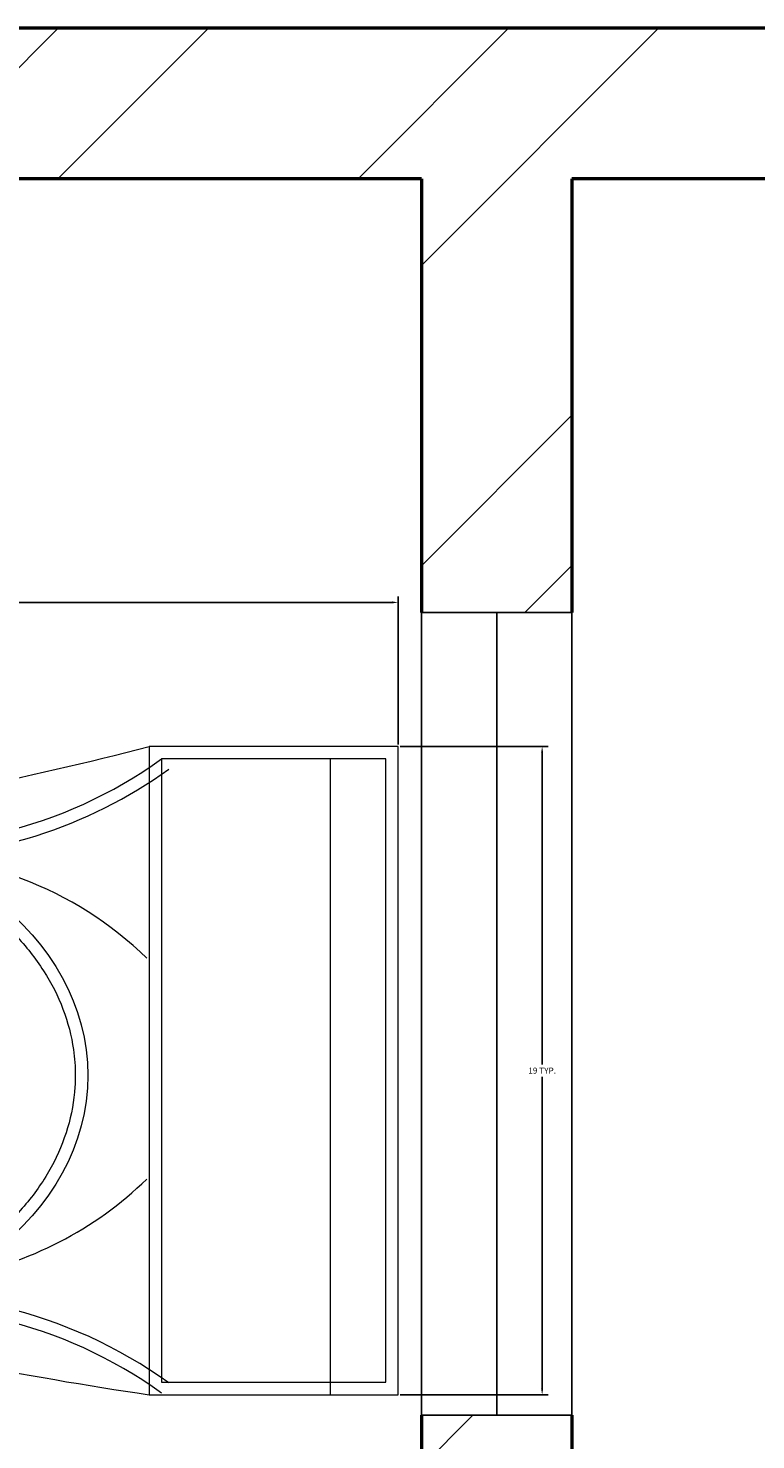
# Model space of a CAD drawing. Units: inches. Extents: x 963 to 2075, y 289 to 2657.
# Tile 35 of 98: x 1668 to 1689, y 1505 to 1547. Entities that reach past the tile are written whole.
import ezdxf

# ---------------------------------------------------------------- set-up
doc = ezdxf.new("R2010")
doc.units = ezdxf.units.IN
for name, color, linetype, lineweight in [('A-ANNO-DIMS', 2, 'Continuous', 18), ('A-FLOR-FIXT', 9, 'Continuous', 18), ('A-GLAZ', 3, 'Continuous', 25), ('A-WALL', 7, 'Continuous', 50), ('A-WALL-PATT', 8, 'Continuous', 13)]:
    doc.layers.add(name, color=color, linetype=linetype, lineweight=lineweight)
doc.styles.get("Standard").update_dxf_attribs({"font": 'arial.ttf'})
doc.dimstyles.get("Standard").update_dxf_attribs({"dimtxt": 0.18, "dimasz": 0.18, "dimexe": 0.18, "dimexo": 0.0625, "dimgap": 0.09, "dimtad": 0, "dimtih": 1, "dimtoh": 1, "dimdec": 4, "dimzin": 0, "dimdsep": 46, "dimtxsty": 'Standard', "dimcen": 0.09, "dimadec": 0, "dimazin": 0, "dimtfac": 1, "dimtdec": 4, "dimtofl": 0, "dimtmove": 0, "dimatfit": 3, "dimfxl": 1, "dimtolj": 1, "dimtzin": 0, "dimarcsym": 0})

# ---------------------------------------------------------------- blocks, each defined once
blk = doc.blocks.new('A$C31115884')
for p, q in [((257.5, 466.4), (257.5, 523.2)), ((283.1, 497.7), (223.4, 497.7)), ((0, 200), (0, 0)), ((520, 200), (0, 200)), ((520, 0), (520, 200)), ((10, 190), (10, 10)), ((510, 190), (10, 190)), ((510, 10), (510, 190)), ((510, 54.5), (0, 54.5)), ((10, 10), (510, 10)), ((0, 0), (520, 0))]:
    blk.add_line(p, q)
blk.add_circle((255.6, 496.4), 23.6)
for centre, radius, start, end in [((2777.7, -204.6), 2807, 165.4549, 171.7133), ((3237, 905), 2807, 188.2867, 194.5451), ((-294.5, 403.3), 364.7, 324.2091, 9.3499), ((-294.5, 403.3), 374.7, 324.2091, 9.3499), ((805.8, 403.3), 364.7, 170.6501, 215.7909), ((139.5, 406.2), 293.5, 315.8436, 2.6563), ((805.8, 403.3), 374.7, 179.2036, 215.7909), ((383.6, 406.2), 293.5, 190.2774, 224.1564)]:
    blk.add_arc(centre, radius, start, end)
blk.add_ellipse((256.2, 509.9), major_axis=(0, -260.7), ratio=0.772727)
blk.add_open_spline([(256.2, 259.2), (263.1, 259.2), (270, 259.7), (287.8, 262.3), (298.7, 265.1), (319.9, 273.1), (330.2, 278.4), (350.1, 291.1), (359.7, 298.7), (377.7, 315.9), (386.2, 325.5), (401.7, 346.6), (408.8, 358.1), (421.3, 382.5), (426.8, 395.5), (435.9, 422.4), (439.5, 436.4), (444.8, 465.1), (446.5, 479.7), (447.9, 509.2), (447.6, 524), (445, 553.3), (442.7, 567.8), (436.3, 596), (432.1, 609.7), (421.9, 636), (416, 648.6), (402.5, 672.1), (395, 683), (378.6, 703), (369.8, 712.1), (351.1, 728), (341.3, 734.8), (320.9, 746.2), (310.4, 750.7), (288.9, 757.3), (278, 759.4), (256, 761), (245, 760.6), (223.1, 757.2), (212.3, 754.3), (191.1, 746.1), (180.8, 740.7), (160.9, 727.8), (151.4, 720.1), (133.5, 702.7), (125.1, 693), (109.6, 671.7), (102.6, 660.2), (90.2, 635.7), (84.9, 622.7), (76, 595.6), (72.4, 581.6), (67.2, 552.9), (65.6, 538.2), (64.4, 508.8), (64.8, 494), (67.5, 464.7), (69.9, 450.2), (76.6, 422), (80.8, 408.3), (91.1, 382.2), (97.2, 369.7), (110.8, 346.3), (118.4, 335.4), (134.8, 315.6), (143.7, 306.7), (162.4, 290.9), (172.3, 284.2), (192.8, 273), (203.3, 268.6), (224.8, 262.2), (235.8, 260.2), (249.9, 259.3), (253, 259.2), (256.2, 259.2)], degree=3, knots=[0, 0, 0, 0, 0.110105, 0.110105, 0.285049, 0.285049, 0.459994, 0.459994, 0.634938, 0.634938, 0.809882, 0.809882, 0.984827, 0.984827, 1.159771, 1.159771, 1.334715, 1.334715, 1.50966, 1.50966, 1.684604, 1.684604, 1.859549, 1.859549, 2.034493, 2.034493, 2.209437, 2.209437, 2.384382, 2.384382, 2.559326, 2.559326, 2.73427, 2.73427, 2.909215, 2.909215, 3.084159, 3.084159, 3.259103, 3.259103, 3.434048, 3.434048, 3.608992, 3.608992, 3.783936, 3.783936, 3.958881, 3.958881, 4.133825, 4.133825, 4.30877, 4.30877, 4.483714, 4.483714, 4.658658, 4.658658, 4.833603, 4.833603, 5.008547, 5.008547, 5.183491, 5.183491, 5.358436, 5.358436, 5.53338, 5.53338, 5.708324, 5.708324, 5.883269, 5.883269, 6.058213, 6.058213, 6.233158, 6.233158, 6.283185, 6.283185, 6.283185, 6.283185])
blk = doc.blocks.new('*D16')
at = {"layer": 'A-ANNO-DIMS', "color": 0, "lineweight": -2, "transparency": 16777216}
for p, q in [((1650.002, 1525.905), (1650.002, 1530.33)), ((1678.722, 1525.905), (1678.722, 1530.33)), ((1650.182, 1530.15), (1663.586, 1530.15)), ((1678.542, 1530.15), (1665.138, 1530.15))]:
    blk.add_line(p, q, dxfattribs=at)
at = {"layer": 'A-ANNO-DIMS', "color": 0, "transparency": 16777216}
for points in [[(1650.182, 1530.18), (1650.182, 1530.12), (1650.002, 1530.15)], [(1678.542, 1530.18), (1678.542, 1530.12), (1678.722, 1530.15)]]:
    blk.add_solid(points, dxfattribs=at)
at = {"layer": 'Defpoints', "color": 0, "transparency": 16777216}
for p in [(1650.002, 1530.15), (1650.002, 1525.842), (1678.722, 1525.842)]:
    blk.add_point(p, dxfattribs=at)
at = {"layer": 'A-ANNO-DIMS', "color": 0, "transparency": 16777216, "insert": (1664.362, 1530.15), "char_height": 0.18, "attachment_point": 5}
blk.add_mtext('\\A1;WC 29 TYP.', dxfattribs=at)
blk = doc.blocks.new('*D17')
at = {"layer": 'A-ANNO-DIMS', "color": 0, "lineweight": -2, "transparency": 16777216}
for p, q in [((1678.785, 1525.842), (1683.21, 1525.842)), ((1683.03, 1525.662), (1683.03, 1516.334)), ((1683.03, 1506.641), (1683.03, 1515.97)), ((1678.785, 1506.461), (1683.21, 1506.461))]:
    blk.add_line(p, q, dxfattribs=at)
at = {"layer": 'A-ANNO-DIMS', "color": 0, "transparency": 16777216}
for points in [[(1683, 1525.662), (1683.06, 1525.662), (1683.03, 1525.842)], [(1683, 1506.641), (1683.06, 1506.641), (1683.03, 1506.461)]]:
    blk.add_solid(points, dxfattribs=at)
at = {"layer": 'Defpoints', "color": 0, "transparency": 16777216}
for p in [(1678.722, 1525.842), (1683.03, 1525.842), (1678.722, 1506.461)]:
    blk.add_point(p, dxfattribs=at)
at = {"layer": 'A-ANNO-DIMS', "color": 0, "transparency": 16777216, "insert": (1683.03, 1516.152), "char_height": 0.18, "attachment_point": 5}
blk.add_mtext('\\A1;19 TYP.', dxfattribs=at)

msp = doc.modelspace()

# ---------------------------------------------------------------- hatches: boundary and pattern name
at = {"layer": 'A-WALL-PATT'}
h = msp.add_hatch(dxfattribs=at)
h.set_pattern_fill('ANSI32', color=256)
h.paths.add_polyline_path([(1910.422, 1929.422), (1910.422, 1963.511), (1905.922, 1963.511), (1905.922, 1929.422), (1845.922, 1929.422), (1845.922, 1993.365), (1843.672, 1993.365), (1841.422, 1993.365), (1841.422, 1951.163), (1841.422, 1924.922), (1853.422, 1924.922), (1853.422, 1913.074), (1857.922, 1913.074), (1857.922, 1924.922), (1910.422, 1924.922)])
h.paths.add_polyline_path([(1857.922, 1853.074), (1853.422, 1853.074), (1853.422, 1826.318), (1841.422, 1826.318), (1674.482, 1826.318), (1674.482, 1821.818), (1853.422, 1821.818), (1857.922, 1821.818)])
h.paths.add_polyline_path([(1857.922, 1821.818), (1853.422, 1821.818), (1853.422, 1807.793), (1857.922, 1807.793)])
h.paths.add_polyline_path([(1857.922, 1747.793), (1853.422, 1747.793), (1853.422, 1713.818), (1809.343, 1713.818), (1809.343, 1709.318), (1905.922, 1709.318), (1905.922, 1688.318), (1910.422, 1688.318), (1910.422, 1713.818), (1857.922, 1713.818)])
h.paths.add_polyline_path([(1830.922, 1542.818), (1837.429, 1542.818), (1837.429, 1545.068), (1837.429, 1547.318), (1823.419, 1547.318), (1823.419, 1545.068), (1823.419, 1542.818), (1826.422, 1542.818), (1826.422, 1482.818), (1742.422, 1482.818), (1742.422, 1505.389), (1737.922, 1505.389), (1737.922, 1478.318), (1830.922, 1478.318)])
h.paths.add_polyline_path([(1938.922, 1619.318), (1934.422, 1619.318), (1910.422, 1619.318), (1910.422, 1628.318), (1908.172, 1628.318), (1905.922, 1628.318), (1905.922, 1614.818), (1934.422, 1614.818), (1934.422, 1547.318), (1905.922, 1547.318), (1899.589, 1547.318), (1899.589, 1542.818), (1910.422, 1542.818), (1938.922, 1542.818)])
h.paths.add_polyline_path([(1803.676, 1547.318), (1773.922, 1547.318), (1773.922, 1709.318), (1777.757, 1709.318), (1777.757, 1713.818), (1701.922, 1713.818), (1701.922, 1697.802), (1706.422, 1697.802), (1706.422, 1709.318), (1769.422, 1709.318), (1769.422, 1662.818), (1706.422, 1662.818), (1706.422, 1674.385), (1701.922, 1674.385), (1701.922, 1662.818), (1675.672, 1662.818), (1675.672, 1658.318), (1769.422, 1658.318), (1769.422, 1547.318), (1729.17, 1547.318), (1729.17, 1542.818), (1737.922, 1542.818), (1737.922, 1529.389), (1742.422, 1529.389), (1742.422, 1542.818), (1803.676, 1542.818)])
h.paths.add_polyline_path([(1595.422, 1542.818), (1599.245, 1542.818), (1599.245, 1547.318), (1584.36, 1547.318), (1584.36, 1542.818), (1590.922, 1542.818), (1590.922, 1436.318), (1595.422, 1436.318), (1595.422, 1440.818)])
h.paths.add_polyline_path([(1693.17, 1547.318), (1649.422, 1547.318), (1649.422, 1658.318), (1652.098, 1658.318), (1652.098, 1660.568), (1652.098, 1662.818), (1649.422, 1662.818), (1649.422, 1680.937), (1647.172, 1680.937), (1644.922, 1680.937), (1644.922, 1547.318), (1622.422, 1547.318), (1622.422, 1545.068), (1622.422, 1542.818), (1649.422, 1542.818), (1679.422, 1542.818), (1679.422, 1529.845), (1681.672, 1529.845), (1683.922, 1529.845), (1683.922, 1542.818), (1693.17, 1542.818), (1693.17, 1545.068)])
h.paths.add_polyline_path([(1683.922, 1505.845), (1679.422, 1505.845), (1679.422, 1483.805), (1595.422, 1483.805), (1595.422, 1479.305), (1683.922, 1479.305)])
h.paths.add_polyline_path([(1402.993, 1547.318), (1376.422, 1547.318), (1376.422, 1675.888), (1374.172, 1675.888), (1371.922, 1675.888), (1371.922, 1662.818), (1368.876, 1662.818), (1368.876, 1658.318), (1371.922, 1658.318), (1371.922, 1547.318), (1335.464, 1547.318), (1335.464, 1542.818), (1337.422, 1542.818), (1337.422, 1526.732), (1341.922, 1526.732), (1341.922, 1542.818), (1371.922, 1542.818), (1402.993, 1542.818)])

# ---------------------------------------------------------------- linework, layer by layer
at = {"layer": 'A-GLAZ'}
for p, q in [((1683.922, 1529.845), (1679.422, 1529.845)), ((1679.422, 1529.845), (1681.672, 1529.845)), ((1679.422, 1529.845), (1679.422, 1505.845)), ((1681.672, 1529.845), (1681.672, 1505.845)), ((1683.922, 1529.845), (1683.922, 1505.845)), ((1681.672, 1505.845), (1679.422, 1505.845)), ((1679.422, 1505.845), (1683.922, 1505.845))]:
    msp.add_line(p, q, dxfattribs=at)
at = {"layer": 'A-WALL'}
for p, q in [((1693.17, 1547.318), (1649.422, 1547.318)), ((1679.422, 1542.818), (1649.422, 1542.818)), ((1679.422, 1542.818), (1679.422, 1529.845)), ((1683.922, 1542.818), (1683.922, 1529.845)), ((1693.17, 1542.818), (1683.922, 1542.818)), ((1679.422, 1505.845), (1679.422, 1483.805)), ((1683.922, 1505.845), (1683.922, 1479.305))]:
    msp.add_line(p, q, dxfattribs=at)

# ---------------------------------------------------------------- block references
at = {"layer": 'A-FLOR-FIXT', "xscale": 0.0372717239612423, "yscale": 0.0372717239612423, "zscale": 0.0372717239612423, "rotation": 89.99999999999999}
msp.add_blockref('A$C31115884', (1678.722, 1506.461), dxfattribs=at)

# ---------------------------------------------------------------- dimensions: what is measured, and where the dimension line sits
at = {"layer": 'A-ANNO-DIMS'}
for base, p1, p2, angle, text, picture, middle in [((1650.002, 1530.15), (1678.722, 1525.842), (1650.002, 1525.842), 180, 'WC <> TYP.', '*D16', (1664.362, 1530.15)), ((1683.03, 1525.842), (1678.722, 1506.461), (1678.722, 1525.842), 90, '<> TYP.', '*D17', (1683.03, 1516.152))]:
    dim = msp.add_linear_dim(base=base, p1=p1, p2=p2, angle=angle, text=text, dimstyle='Standard', override={"dimdec": 0, "dimlfac": 1, "dimrnd": 0, "dimzin": 0, "dimdsep": 46, "dimlunit": 2}, dxfattribs=at)
    dim.commit()
    dim.dimension.update_dxf_attribs({"geometry": picture, "text_midpoint": middle})

doc.saveas('drawing.dxf')
